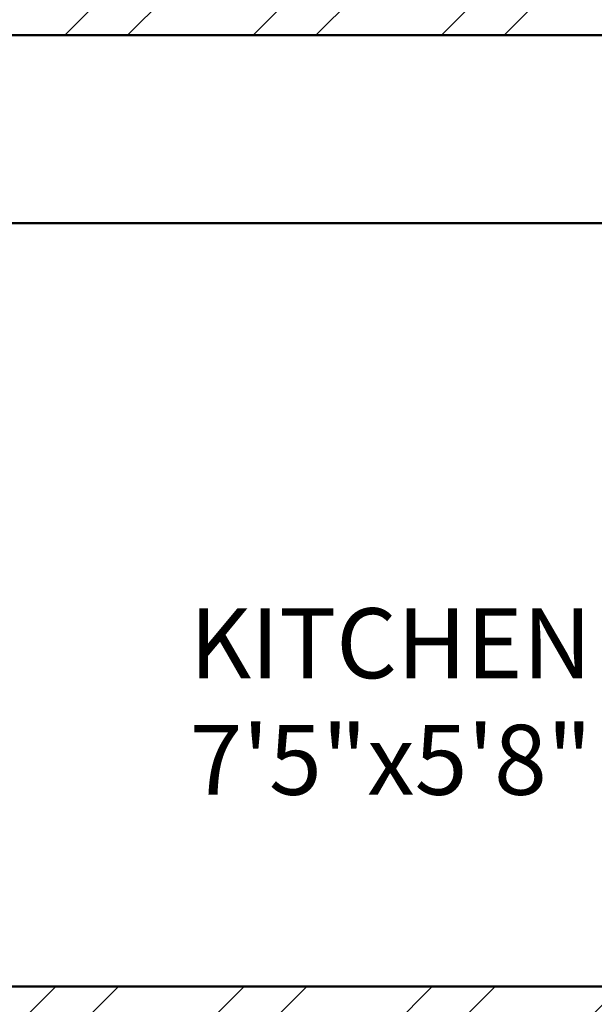
# Model space of a CAD drawing. Units: inches. Extents: x 1901 to 2863, y 888 to 2433.
# Tile 85 of 91: x 2682 to 2723, y 2009 to 2080. Entities that reach past the tile are written whole.
import ezdxf

# ---------------------------------------------------------------- set-up
doc = ezdxf.new("R2010")
doc.units = ezdxf.units.IN
for name, color, linetype, lineweight in [('A-AREA-IDEN', 7, 'Continuous', 18), ('A-WALL', 7, 'Continuous', 50), ('A-WALL-PATT', 8, 'Continuous', 13)]:
    doc.layers.add(name, color=color, linetype=linetype, lineweight=lineweight)
doc.styles.get("Standard").update_dxf_attribs({"font": 'arial.ttf'})

msp = doc.modelspace()

# ---------------------------------------------------------------- hatches: boundary and pattern name
at = {"layer": 'A-WALL-PATT'}
h = msp.add_hatch(dxfattribs=at)
h.set_pattern_fill('ANSI32', color=256)
h.paths.add_polyline_path([(2192.501, 2274.134), (2141.264, 2274.134), (2141.264, 2269.634), (2192.501, 2269.634)])
h.paths.add_polyline_path([(2259.926, 2274.134), (2216.501, 2274.134), (2216.501, 2269.634), (2255.426, 2269.634), (2255.426, 2214.634), (2250.809, 2214.634), (2250.809, 2210.134), (2259.926, 2210.134), (2259.926, 2215.134), (2271.756, 2215.134), (2271.756, 2217.384), (2271.756, 2219.634), (2259.926, 2219.634)])
h.paths.add_polyline_path([(2171.426, 2269.634), (2166.926, 2269.634), (2166.926, 2219.634), (2121.238, 2219.634), (2121.238, 2215.134), (2166.926, 2215.134), (2166.926, 2083.134), (2161.807, 2083.134), (2161.807, 2078.634), (2171.426, 2078.634), (2176.996, 2078.634), (2176.996, 2080.884), (2176.996, 2083.134), (2171.426, 2083.134), (2171.426, 2210.134), (2230.912, 2210.134), (2230.912, 2212.384), (2230.912, 2214.634), (2171.426, 2214.634)])
h.paths.add_polyline_path([(2117.264, 2274.134), (2089.426, 2274.134), (2089.426, 2219.634), (2081.136, 2219.634), (2081.136, 2215.134), (2089.426, 2215.134), (2098.004, 2215.134), (2098.004, 2217.384), (2098.004, 2219.634), (2093.926, 2219.634), (2093.926, 2269.634), (2117.264, 2269.634), (2117.264, 2271.884)])
h.paths.add_polyline_path([(2343.426, 2219.634), (2329.295, 2219.634), (2329.295, 2215.134), (2338.926, 2215.134), (2338.926, 2184.739), (2343.426, 2184.739)])
h.paths.add_polyline_path([(2338.926, 2083.134), (2329.295, 2083.134), (2208.966, 2083.134), (2208.966, 2078.634), (2338.926, 2078.634)])
h.paths.add_polyline_path([(2343.426, 2136.739), (2338.926, 2136.739), (2338.926, 1872.634), (2343.426, 1872.634)])
h.paths.add_polyline_path([(2343.426, 1863.634), (2397.68, 1863.634), (2397.68, 1821.634), (2384.138, 1821.634), (2384.138, 1812.634), (2418.33, 1812.634), (2418.33, 1817.134), (2418.33, 1821.634), (2406.68, 1821.634), (2406.68, 1863.634), (2459.499, 1863.634), (2459.499, 1821.634), (2447.138, 1821.634), (2447.138, 1812.634), (2459.499, 1812.634), (2468.499, 1812.634), (2468.499, 1872.634), (2394.426, 1872.634), (2334.426, 1872.634), (2334.426, 1812.634), (2343.426, 1812.634), (2353.251, 1812.634), (2353.251, 1821.634), (2343.426, 1821.634)])
h.paths.add_polyline_path([(2510.014, 1872.634), (2468.499, 1872.634), (2468.499, 1868.134), (2510.014, 1868.134)])
h.paths.add_polyline_path([(2514.009, 1817.134), (2468.499, 1817.134), (2468.499, 1812.634), (2482.114, 1812.634), (2482.114, 1800.606), (2486.614, 1800.606), (2486.614, 1812.634), (2514.009, 1812.634)])
h.paths.add_polyline_path([(2299.247, 1814.884), (2299.247, 1817.134), (2295.926, 1817.134), (2295.926, 1854.169), (2293.676, 1854.169), (2291.426, 1854.169), (2291.426, 1817.134), (2266.109, 1817.134), (2266.109, 1812.634), (2299.247, 1812.634)])
h.paths.add_polyline_path([(2218.109, 1817.134), (2206.46, 1817.134), (2171.426, 1817.134), (2171.426, 1949.134), (2190.1, 1949.134), (2190.1, 1953.634), (2163.468, 1953.634), (2163.468, 1949.134), (2166.926, 1949.134), (2166.926, 1817.134), (2114.297, 1817.134), (2114.297, 1812.634), (2218.109, 1812.634)])
h.paths.add_polyline_path([(2029.426, 1970.922), (2024.926, 1970.922), (2024.926, 1912.717), (2029.426, 1912.717)])
h.paths.add_polyline_path([(2132.297, 1953.634), (2113.926, 1953.634), (2113.926, 1975.888), (2111.676, 1975.888), (2109.426, 1975.888), (2109.426, 1953.634), (2029.426, 1953.634), (2029.426, 1949.134), (2132.297, 1949.134)])
h.paths.add_polyline_path([(2029.426, 1853.606), (2029.31, 1853.606), (2029.31, 1853.606), (2029.426, 1853.606), (2029.426, 1864.717), (2024.926, 1864.717), (2024.926, 1812.634), (2066.297, 1812.634), (2066.297, 1814.884), (2066.297, 1817.134), (2029.426, 1817.134)])
h.paths.add_polyline_path([(2122.926, 2010.088), (2120.676, 2010.088), (2118.426, 2010.088), (2118.426, 2006.134), (2029.426, 2006.134), (2029.426, 2001.634), (2109.426, 2001.634), (2109.426, 1998.041), (2113.926, 1998.041), (2113.926, 2001.634), (2122.926, 2001.634)])
h.paths.add_polyline_path([(2029.426, 2031.376), (2024.926, 2031.376), (2024.926, 1994.922), (2027.176, 1994.922), (2029.426, 1994.922)])
h.paths.add_polyline_path([(2029.426, 2136.739), (2024.926, 2136.739), (2024.926, 2067.376), (2027.176, 2067.376), (2029.426, 2067.376)])
h.paths.add_polyline_path([(2125.618, 2083.134), (2029.426, 2083.134), (2029.426, 2078.634), (2118.426, 2078.634), (2118.426, 2030.715), (2122.926, 2030.715), (2122.926, 2078.634), (2125.618, 2078.634)])
h.paths.add_polyline_path([(2029.426, 2215.134), (2040.468, 2215.134), (2040.468, 2217.384), (2040.468, 2219.634), (2024.926, 2219.634), (2024.926, 2184.739), (2029.426, 2184.739), (2029.426, 2187.778)])
h.paths.add_polyline_path([(2686.426, 2274.134), (2659.284, 2274.134), (2659.284, 2269.634), (2681.926, 2269.634), (2681.926, 2219.634), (2676.816, 2219.634), (2676.816, 2215.134), (2681.926, 2215.134), (2697.011, 2215.134), (2697.011, 2217.384), (2697.011, 2219.634), (2686.426, 2219.634)])
h.paths.add_polyline_path([(2609.926, 2269.634), (2635.284, 2269.634), (2635.284, 2274.134), (2571.431, 2274.134), (2571.431, 2269.634), (2605.426, 2269.634), (2605.426, 2214.634), (2549.098, 2214.634), (2549.098, 2210.134), (2605.426, 2210.134), (2605.426, 2083.134), (2601.014, 2083.134), (2601.014, 2080.884), (2601.014, 2078.634), (2609.926, 2078.634), (2616.162, 2078.634), (2616.162, 2080.884), (2616.162, 2083.134), (2609.926, 2083.134), (2609.926, 2215.134), (2651.465, 2215.134), (2651.465, 2217.384), (2651.465, 2219.634), (2609.926, 2219.634)])
h.paths.add_polyline_path([(2521.426, 2269.634), (2547.431, 2269.634), (2547.431, 2271.884), (2547.431, 2274.134), (2516.926, 2274.134), (2516.926, 2219.634), (2506.41, 2219.634), (2506.41, 2215.134), (2516.926, 2215.134), (2516.926, 2210.134), (2525.402, 2210.134), (2525.402, 2212.384), (2525.402, 2214.634), (2521.426, 2214.634)])
h.paths.add_polyline_path([(2456.011, 2219.634), (2439.426, 2219.634), (2439.426, 2187.888), (2443.926, 2187.888), (2443.926, 2215.134), (2456.011, 2215.134)])
h.paths.add_polyline_path([(2752.926, 2219.634), (2739.485, 2219.634), (2739.485, 2215.134), (2748.426, 2215.134), (2748.426, 2187.888), (2752.926, 2187.888)])
h.paths.add_polyline_path([(2752.926, 2139.888), (2748.426, 2139.888), (2748.426, 2083.134), (2648.416, 2083.134), (2648.416, 2078.634), (2654.926, 2078.634), (2654.926, 2039.437), (2659.426, 2039.437), (2659.426, 2078.634), (2748.426, 2078.634), (2748.426, 2063.429), (2752.926, 2063.429)])
h.paths.add_polyline_path([(2752.926, 2010.634), (2659.426, 2010.634), (2659.426, 2015.652), (2654.926, 2015.652), (2654.926, 2010.634), (2605.426, 2010.634), (2605.426, 1920.967), (2609.926, 1920.967), (2609.926, 2006.134), (2748.426, 2006.134), (2748.426, 1982.466), (2752.926, 1982.466)])
h.paths.add_polyline_path([(2752.926, 2027.429), (2748.426, 2027.429), (2748.426, 2010.634), (2752.926, 2010.634)])
h.paths.add_polyline_path([(2748.426, 1886.134), (2609.926, 1886.134), (2609.926, 1889.719), (2605.426, 1889.719), (2605.426, 1861.262), (2609.926, 1861.262), (2609.926, 1881.634), (2748.426, 1881.634)])
h.paths.add_polyline_path([(2456.855, 2228.831), (2498.401, 2228.831), (2498.401, 2247.488), (2456.855, 2247.488)], flags=9)
h.paths.add_polyline_path([(2038.602, 2237.418), (2080.174, 2237.418), (2080.174, 2256.075), (2038.602, 2256.075)], flags=9)
h.paths.add_polyline_path([(2292.009, 1062.394), (2539.932, 1062.394), (2539.932, 1099.487), (2292.009, 1099.487)], flags=9)
h.paths.add_polyline_path([(2424.91, 1832.253), (2448.513, 1832.253), (2448.513, 1846.678), (2424.91, 1846.678)], flags=25)
h.paths.add_polyline_path([(2359.076, 1832.253), (2382.678, 1832.253), (2382.678, 1846.678), (2359.076, 1846.678)], flags=25)
h.paths.add_polyline_path([(2352.899, 1684.802), (2367.543, 1684.802), (2367.543, 1697.167), (2352.899, 1697.167)], flags=9)
h.paths.add_polyline_path([(2079.288, 1755.826), (2169.024, 1755.826), (2169.024, 1774.372), (2079.288, 1774.372)], flags=9)
h.paths.add_polyline_path([(2404.09, 1373.857), (2404.09, 1463.593), (2385.544, 1463.593), (2385.544, 1373.857)], flags=9)
h.paths.add_polyline_path([(2268.091, 2236.371), (2309.636, 2236.371), (2309.636, 2255.028), (2268.091, 2255.028)], flags=9)
h.paths.add_polyline_path([(2575.96, 1700.951), (2665.696, 1700.951), (2665.696, 1719.498), (2575.96, 1719.498)], flags=9)
h.paths.add_polyline_path([(2302.962, 1878.474), (2329.524, 1878.474), (2329.524, 1888.777), (2302.962, 1888.777)], flags=9)
h.paths.add_polyline_path([(2097.415, 2240.576), (2126.573, 2240.576), (2126.573, 2259.233), (2097.415, 2259.233)], flags=9)
h.paths.add_polyline_path([(2208.725, 2246.124), (2237.882, 2246.124), (2237.882, 2264.781), (2208.725, 2264.781)], flags=9)
h.paths.add_polyline_path([(2038.147, 1925.958), (2076.987, 1925.958), (2076.987, 1944.615), (2038.147, 1944.615)], flags=9)
h.paths.add_polyline_path([(2239.144, 1926.672), (2288.465, 1926.672), (2288.465, 1945.329), (2239.144, 1945.329)], flags=9)
h.paths.add_polyline_path([(2175.429, 2007.33), (2212.356, 2007.33), (2212.356, 2025.987), (2175.429, 2025.987)], flags=9)
h.paths.add_polyline_path([(2225.034, 2091.794), (2263.875, 2091.794), (2263.875, 2110.451), (2225.034, 2110.451)], flags=9)
h.paths.add_polyline_path([(2035.398, 2098.478), (2074.238, 2098.478), (2074.238, 2117.135), (2035.398, 2117.135)], flags=9)
h.paths.add_polyline_path([(2050.102, 2029.209), (2083.26, 2029.209), (2083.26, 2047.866), (2050.102, 2047.866)], flags=9)
h.paths.add_polyline_path([(2069.677, 1956.719), (2098.835, 1956.719), (2098.835, 1975.376), (2069.677, 1975.376)], flags=25)
h.paths.add_polyline_path([(2328.62, 1753.336), (2361.663, 1753.336), (2361.663, 1771.993), (2328.62, 1771.993)], flags=9)
h.paths.add_polyline_path([(2395.162, 2060.888), (2395.162, 2140.654), (2378.676, 2140.654), (2378.676, 2060.888)], flags=9)
h.paths.add_polyline_path([(2463.728, 2059.02), (2492.886, 2059.02), (2492.886, 2077.677), (2463.728, 2077.677)], flags=9)
h.paths.add_polyline_path([(2458.027, 2181.536), (2496.868, 2181.536), (2496.868, 2200.194), (2458.027, 2200.194)], flags=9)
h.paths.add_polyline_path([(2527.577, 2243.074), (2556.735, 2243.074), (2556.735, 2261.731), (2527.577, 2261.731)], flags=9)
h.paths.add_polyline_path([(2694.461, 2232.767), (2736.033, 2232.767), (2736.033, 2251.425), (2694.461, 2251.425)], flags=9)
h.paths.add_polyline_path([(2637.821, 2249.225), (2666.979, 2249.225), (2666.979, 2267.882), (2637.821, 2267.882)], flags=9)
h.paths.add_polyline_path([(2623.687, 2183.541), (2662.528, 2183.541), (2662.528, 2202.199), (2623.687, 2202.199)], flags=9)
h.paths.add_polyline_path([(2691.965, 2021.5), (2725.124, 2021.5), (2725.124, 2040.157), (2691.965, 2040.157)], flags=9)
h.paths.add_polyline_path([(2621.043, 1975.912), (2662.335, 1975.912), (2662.335, 1994.569), (2621.043, 1994.569)], flags=25)
h.paths.add_polyline_path([(2479.032, 1927.62), (2519.844, 1927.62), (2519.844, 1946.277), (2479.032, 1946.277)], flags=9)
h.paths.add_polyline_path([(2670.941, 1849.076), (2716.005, 1849.076), (2716.005, 1867.734), (2670.941, 1867.734)], flags=9)
h.paths.add_polyline_path([(2523.613, 1782.956), (2550.175, 1782.956), (2550.175, 1793.26), (2523.613, 1793.26)], flags=9)
h.paths.add_polyline_path([(2450.841, 1207.331), (2492.386, 1207.331), (2492.386, 1225.989), (2450.841, 1225.989)], flags=9)
h.paths.add_polyline_path([(2527.751, 1203.841), (2556.908, 1203.841), (2556.908, 1222.499), (2527.751, 1222.499)], flags=9)
h.paths.add_polyline_path([(2639.111, 1207.2), (2668.268, 1207.2), (2668.268, 1225.857), (2639.111, 1225.857)], flags=9)
h.paths.add_polyline_path([(2692.594, 1218.965), (2734.167, 1218.965), (2734.167, 1237.623), (2692.594, 1237.623)], flags=9)
h.paths.add_polyline_path([(2669.266, 1366.329), (2708.106, 1366.329), (2708.106, 1384.987), (2669.266, 1384.987)], flags=9)
h.paths.add_polyline_path([(2463.313, 1358.031), (2502.153, 1358.031), (2502.153, 1376.688), (2463.313, 1376.688)], flags=9)
h.paths.add_polyline_path([(2494.725, 1449.963), (2531.652, 1449.963), (2531.652, 1468.62), (2494.725, 1468.62)], flags=9)
h.paths.add_polyline_path([(2675.565, 1422.157), (2708.724, 1422.157), (2708.724, 1440.815), (2675.565, 1440.815)], flags=9)
h.paths.add_polyline_path([(2685.634, 1493.891), (2714.792, 1493.891), (2714.792, 1512.548), (2685.634, 1512.548)], flags=9)
h.paths.add_polyline_path([(2686.805, 1529.913), (2725.645, 1529.913), (2725.645, 1548.57), (2686.805, 1548.57)], flags=9)
h.paths.add_polyline_path([(2503.651, 1537.991), (2552.972, 1537.991), (2552.972, 1556.648), (2503.651, 1556.648)], flags=9)
h.paths.add_polyline_path([(2291.713, 1643.504), (2318.275, 1643.504), (2318.275, 1653.807), (2291.713, 1653.807)], flags=9)
h.paths.add_polyline_path([(2450.626, 1610.52), (2477.189, 1610.52), (2477.189, 1620.824), (2450.626, 1620.824)], flags=9)
h.paths.add_polyline_path([(2359.985, 1551.814), (2422.253, 1551.814), (2422.253, 1562.117), (2359.985, 1562.117)], flags=9)
h.paths.add_polyline_path([(2280.106, 1249.006), (2321.651, 1249.006), (2321.651, 1267.663), (2280.106, 1267.663)], flags=9)
h.paths.add_polyline_path([(2164.057, 1274.232), (2193.215, 1274.232), (2193.215, 1292.889), (2164.057, 1292.889)], flags=9)
h.paths.add_polyline_path([(2118.21, 1277.694), (2151.252, 1277.694), (2151.252, 1296.351), (2118.21, 1296.351)], flags=9)
h.paths.add_polyline_path([(2031.946, 1268.529), (2073.519, 1268.529), (2073.519, 1287.187), (2031.946, 1287.187)], flags=9)
h.paths.add_polyline_path([(2050.199, 1409.079), (2089.04, 1409.079), (2089.04, 1427.736), (2050.199, 1427.736)], flags=9)
h.paths.add_polyline_path([(2243.743, 1421.032), (2282.584, 1421.032), (2282.584, 1439.689), (2243.743, 1439.689)], flags=9)
h.paths.add_polyline_path([(2190.746, 1509.769), (2231.558, 1509.769), (2231.558, 1528.426), (2190.746, 1528.426)], flags=9)
h.paths.add_polyline_path([(2058.392, 1475.415), (2091.55, 1475.415), (2091.55, 1494.073), (2058.392, 1494.073)], flags=9)
h.paths.add_polyline_path([(2062.447, 1553.09), (2091.605, 1553.09), (2091.605, 1571.747), (2062.447, 1571.747)], flags=9)
h.paths.add_polyline_path([(2219.524, 1590.365), (2266.147, 1590.365), (2266.147, 1609.022), (2219.524, 1609.022)], flags=9)
h.paths.add_polyline_path([(2041.072, 1584.188), (2079.912, 1584.188), (2079.912, 1602.845), (2041.072, 1602.845)], flags=9)
h = msp.add_hatch(dxfattribs=at)
h.set_pattern_fill('ANSI32', color=256)
h.paths.add_polyline_path([(2443.926, 2139.888), (2439.426, 2139.888), (2439.426, 2069.348), (2441.676, 2069.348), (2443.926, 2069.348), (2443.926, 2078.634), (2521.926, 2078.634), (2521.926, 2075.067), (2524.176, 2075.067), (2526.426, 2075.067), (2526.426, 2078.634), (2571.755, 2078.634), (2571.755, 2080.884), (2571.755, 2083.134), (2443.926, 2083.134)])
h.paths.add_polyline_path([(2526.426, 2054.634), (2524.176, 2054.634), (2521.926, 2054.634), (2521.926, 2030.634), (2443.926, 2030.634), (2443.926, 2045.348), (2439.426, 2045.348), (2439.426, 1983.867), (2443.926, 1983.867), (2443.926, 2026.134), (2521.926, 2026.134), (2526.426, 2026.134)])
h.paths.add_polyline_path([(2443.926, 1923.867), (2439.426, 1923.867), (2439.426, 1872.634), (2443.926, 1872.634)])
h.paths.add_polyline_path([(2636.233, 1766.134), (2609.926, 1766.134), (2609.926, 1779.785), (2605.426, 1779.785), (2605.426, 1766.134), (2486.614, 1766.134), (2486.614, 1770.671), (2482.114, 1770.671), (2482.114, 1766.134), (2482.114, 1761.634), (2636.233, 1761.634), (2636.233, 1763.884)])
h.paths.add_polyline_path([(2519.536, 1663.384), (2519.536, 1665.634), (2494.926, 1665.634), (2481.831, 1665.634), (2481.831, 1663.384), (2481.831, 1661.134), (2490.426, 1661.134), (2490.426, 1640.157), (2494.926, 1640.157), (2494.926, 1661.134), (2519.536, 1661.134)])
h.paths.add_polyline_path([(2443.926, 1712.134), (2443.926, 1716.634), (2414.464, 1716.634), (2414.464, 1712.134), (2439.426, 1712.134), (2439.426, 1545.507), (2443.926, 1545.507), (2443.926, 1661.134), (2448.475, 1661.134), (2448.475, 1665.634), (2443.926, 1665.634)])
h.paths.add_polyline_path([(2343.426, 1712.134), (2365.525, 1712.134), (2365.525, 1714.384), (2365.525, 1716.634), (2333.871, 1716.634), (2333.871, 1714.384), (2333.871, 1712.134), (2338.926, 1712.134), (2338.926, 1575.634), (2338.926, 1545.507), (2343.426, 1545.507), (2343.426, 1547.507), (2343.426, 1580.134)])
h.paths.add_polyline_path([(2752.926, 1665.634), (2579.536, 1665.634), (2579.536, 1661.134), (2615.926, 1661.134), (2615.926, 1529.134), (2598.931, 1529.134), (2598.931, 1524.634), (2623.127, 1524.634), (2623.127, 1526.884), (2623.127, 1529.134), (2620.426, 1529.134), (2620.426, 1661.134), (2748.426, 1661.134), (2748.426, 1633.499), (2752.926, 1633.499)])
h.paths.add_polyline_path([(2752.926, 1419.929), (2748.426, 1419.929), (2748.426, 1400.134), (2659.426, 1400.134), (2659.426, 1444.333), (2657.176, 1444.333), (2654.926, 1444.333), (2654.926, 1400.134), (2643.649, 1400.134), (2643.649, 1395.634), (2748.426, 1395.634), (2748.426, 1364.035), (2752.926, 1364.035)])
h.paths.add_polyline_path([(2752.926, 1492.878), (2748.426, 1492.878), (2748.426, 1476.634), (2667.426, 1476.634), (2667.426, 1479.71), (2665.176, 1479.71), (2662.926, 1479.71), (2662.926, 1476.634), (2654.926, 1476.634), (2654.926, 1469.536), (2659.426, 1469.536), (2659.426, 1472.134), (2748.426, 1472.134), (2748.426, 1455.929), (2752.926, 1455.929)])
h.paths.add_polyline_path([(2752.926, 1304.035), (2748.426, 1304.035), (2748.426, 1263.634), (2738.66, 1263.634), (2738.66, 1259.134), (2752.926, 1259.134)])
h.paths.add_polyline_path([(2685.926, 1259.134), (2695.49, 1259.134), (2695.49, 1261.384), (2695.49, 1263.634), (2677.837, 1263.634), (2677.837, 1261.384), (2677.837, 1259.134), (2681.426, 1259.134), (2681.426, 1203.634), (2653.277, 1203.634), (2653.277, 1199.134), (2685.926, 1199.134), (2685.926, 1203.634)])
h.paths.add_polyline_path([(2609.426, 1395.634), (2611.848, 1395.634), (2611.848, 1400.134), (2598.888, 1400.134), (2598.888, 1397.884), (2598.888, 1395.634), (2604.926, 1395.634), (2604.926, 1268.134), (2554.726, 1268.134), (2554.726, 1265.884), (2554.726, 1263.634), (2604.926, 1263.634), (2604.926, 1203.634), (2571.306, 1203.634), (2571.306, 1199.134), (2604.926, 1199.134), (2629.277, 1199.134), (2629.277, 1201.384), (2629.277, 1203.634), (2609.426, 1203.634), (2609.426, 1258.634), (2609.426, 1259.134), (2654.804, 1259.134), (2654.804, 1263.634), (2609.426, 1263.634)])
h.paths.add_polyline_path([(2443.926, 1304.035), (2439.426, 1304.035), (2439.426, 1259.134), (2443.926, 1259.134), (2456.16, 1259.134), (2456.16, 1261.384), (2456.16, 1263.634), (2443.926, 1263.634)])
h.paths.add_polyline_path([(2525.426, 1263.634), (2531.778, 1263.634), (2531.778, 1268.134), (2520.926, 1268.134), (2520.926, 1263.634), (2511.409, 1263.634), (2511.409, 1259.134), (2520.926, 1259.134), (2520.926, 1199.134), (2547.306, 1199.134), (2547.306, 1201.384), (2547.306, 1203.634), (2525.426, 1203.634)])
h.paths.add_polyline_path([(2443.926, 1434.842), (2439.426, 1434.842), (2439.426, 1364.035), (2441.676, 1364.035), (2443.926, 1364.035)])
h.paths.add_polyline_path([(2567.134, 1400.134), (2443.926, 1400.134), (2443.926, 1395.634), (2567.134, 1395.634)])
h.paths.add_polyline_path([(2443.926, 1545.507), (2439.426, 1545.507), (2439.426, 1494.842), (2443.926, 1494.842)])
h.paths.add_polyline_path([(2494.926, 1553.349), (2492.676, 1553.349), (2490.426, 1553.349), (2490.426, 1524.634), (2494.926, 1524.634), (2525.936, 1524.634), (2525.936, 1526.884), (2525.936, 1529.134), (2494.926, 1529.134)])
h.paths.add_polyline_path([(2752.926, 1573.499), (2748.426, 1573.499), (2748.426, 1529.134), (2657.759, 1529.134), (2657.759, 1524.634), (2662.926, 1524.634), (2662.926, 1498.631), (2667.426, 1498.631), (2667.426, 1524.634), (2748.426, 1524.634), (2748.426, 1516.878), (2752.926, 1516.878)])
h.paths.add_polyline_path([(2038.602, 2237.418), (2080.174, 2237.418), (2080.174, 2256.075), (2038.602, 2256.075)], flags=9)
h.paths.add_polyline_path([(2292.009, 1062.394), (2539.932, 1062.394), (2539.932, 1099.487), (2292.009, 1099.487)], flags=9)
h.paths.add_polyline_path([(2424.91, 1832.253), (2448.513, 1832.253), (2448.513, 1846.678), (2424.91, 1846.678)], flags=9)
h.paths.add_polyline_path([(2359.076, 1832.253), (2382.678, 1832.253), (2382.678, 1846.678), (2359.076, 1846.678)], flags=9)
h.paths.add_polyline_path([(2352.899, 1684.802), (2367.543, 1684.802), (2367.543, 1697.167), (2352.899, 1697.167)], flags=9)
h.paths.add_polyline_path([(2079.288, 1755.826), (2169.024, 1755.826), (2169.024, 1774.372), (2079.288, 1774.372)], flags=9)
h.paths.add_polyline_path([(2404.09, 1373.857), (2404.09, 1463.593), (2385.544, 1463.593), (2385.544, 1373.857)], flags=9)
h.paths.add_polyline_path([(2268.091, 2236.371), (2309.636, 2236.371), (2309.636, 2255.028), (2268.091, 2255.028)], flags=9)
h.paths.add_polyline_path([(2575.96, 1700.951), (2665.696, 1700.951), (2665.696, 1719.498), (2575.96, 1719.498)], flags=9)
h.paths.add_polyline_path([(2302.962, 1878.474), (2329.524, 1878.474), (2329.524, 1888.777), (2302.962, 1888.777)], flags=9)
h.paths.add_polyline_path([(2097.415, 2240.576), (2126.573, 2240.576), (2126.573, 2259.233), (2097.415, 2259.233)], flags=9)
h.paths.add_polyline_path([(2208.725, 2246.124), (2237.882, 2246.124), (2237.882, 2264.781), (2208.725, 2264.781)], flags=9)
h.paths.add_polyline_path([(2038.147, 1925.958), (2076.987, 1925.958), (2076.987, 1944.615), (2038.147, 1944.615)], flags=9)
h.paths.add_polyline_path([(2239.144, 1926.672), (2288.465, 1926.672), (2288.465, 1945.329), (2239.144, 1945.329)], flags=9)
h.paths.add_polyline_path([(2175.429, 2007.33), (2212.356, 2007.33), (2212.356, 2025.987), (2175.429, 2025.987)], flags=9)
h.paths.add_polyline_path([(2225.034, 2091.794), (2263.875, 2091.794), (2263.875, 2110.451), (2225.034, 2110.451)], flags=9)
h.paths.add_polyline_path([(2035.398, 2098.478), (2074.238, 2098.478), (2074.238, 2117.135), (2035.398, 2117.135)], flags=9)
h.paths.add_polyline_path([(2050.102, 2029.209), (2083.26, 2029.209), (2083.26, 2047.866), (2050.102, 2047.866)], flags=9)
h.paths.add_polyline_path([(2069.677, 1956.719), (2098.835, 1956.719), (2098.835, 1975.376), (2069.677, 1975.376)], flags=9)
h.paths.add_polyline_path([(2328.62, 1753.336), (2361.663, 1753.336), (2361.663, 1771.993), (2328.62, 1771.993)], flags=9)
h.paths.add_polyline_path([(2395.162, 2060.888), (2395.162, 2140.654), (2378.676, 2140.654), (2378.676, 2060.888)], flags=9)
h.paths.add_polyline_path([(2463.728, 2059.02), (2492.886, 2059.02), (2492.886, 2077.677), (2463.728, 2077.677)], flags=9)
h.paths.add_polyline_path([(2458.027, 2181.536), (2496.868, 2181.536), (2496.868, 2200.194), (2458.027, 2200.194)], flags=9)
h.paths.add_polyline_path([(2456.855, 2228.831), (2498.401, 2228.831), (2498.401, 2247.488), (2456.855, 2247.488)], flags=9)
h.paths.add_polyline_path([(2527.577, 2243.074), (2556.735, 2243.074), (2556.735, 2261.731), (2527.577, 2261.731)], flags=9)
h.paths.add_polyline_path([(2694.461, 2232.767), (2736.033, 2232.767), (2736.033, 2251.425), (2694.461, 2251.425)], flags=9)
h.paths.add_polyline_path([(2637.821, 2249.225), (2666.979, 2249.225), (2666.979, 2267.882), (2637.821, 2267.882)], flags=9)
h.paths.add_polyline_path([(2623.687, 2183.541), (2662.528, 2183.541), (2662.528, 2202.199), (2623.687, 2202.199)], flags=9)
h.paths.add_polyline_path([(2691.965, 2021.5), (2725.124, 2021.5), (2725.124, 2040.157), (2691.965, 2040.157)], flags=9)
h.paths.add_polyline_path([(2621.043, 1975.912), (2662.335, 1975.912), (2662.335, 1994.569), (2621.043, 1994.569)], flags=9)
h.paths.add_polyline_path([(2479.032, 1927.62), (2519.844, 1927.62), (2519.844, 1946.277), (2479.032, 1946.277)], flags=9)
h.paths.add_polyline_path([(2670.941, 1849.076), (2716.005, 1849.076), (2716.005, 1867.734), (2670.941, 1867.734)], flags=9)
h.paths.add_polyline_path([(2523.613, 1782.956), (2550.175, 1782.956), (2550.175, 1793.26), (2523.613, 1793.26)], flags=9)
h.paths.add_polyline_path([(2450.841, 1207.331), (2492.386, 1207.331), (2492.386, 1225.989), (2450.841, 1225.989)], flags=9)
h.paths.add_polyline_path([(2527.751, 1203.841), (2556.908, 1203.841), (2556.908, 1222.499), (2527.751, 1222.499)], flags=9)
h.paths.add_polyline_path([(2639.111, 1207.2), (2668.268, 1207.2), (2668.268, 1225.857), (2639.111, 1225.857)], flags=9)
h.paths.add_polyline_path([(2692.594, 1218.965), (2734.167, 1218.965), (2734.167, 1237.623), (2692.594, 1237.623)], flags=9)
h.paths.add_polyline_path([(2669.266, 1366.329), (2708.106, 1366.329), (2708.106, 1384.987), (2669.266, 1384.987)], flags=25)
h.paths.add_polyline_path([(2463.313, 1358.031), (2502.153, 1358.031), (2502.153, 1376.688), (2463.313, 1376.688)], flags=9)
h.paths.add_polyline_path([(2494.725, 1449.963), (2531.652, 1449.963), (2531.652, 1468.62), (2494.725, 1468.62)], flags=9)
h.paths.add_polyline_path([(2675.565, 1422.157), (2708.724, 1422.157), (2708.724, 1440.815), (2675.565, 1440.815)], flags=25)
h.paths.add_polyline_path([(2685.634, 1493.891), (2714.792, 1493.891), (2714.792, 1512.548), (2685.634, 1512.548)], flags=9)
h.paths.add_polyline_path([(2686.805, 1529.913), (2725.645, 1529.913), (2725.645, 1548.57), (2686.805, 1548.57)], flags=25)
h.paths.add_polyline_path([(2503.651, 1537.991), (2552.972, 1537.991), (2552.972, 1556.648), (2503.651, 1556.648)], flags=9)
h.paths.add_polyline_path([(2291.713, 1643.504), (2318.275, 1643.504), (2318.275, 1653.807), (2291.713, 1653.807)], flags=9)
h.paths.add_polyline_path([(2450.626, 1610.52), (2477.189, 1610.52), (2477.189, 1620.824), (2450.626, 1620.824)], flags=9)
h.paths.add_polyline_path([(2359.985, 1551.814), (2422.253, 1551.814), (2422.253, 1562.117), (2359.985, 1562.117)], flags=9)
h.paths.add_polyline_path([(2280.106, 1249.006), (2321.651, 1249.006), (2321.651, 1267.663), (2280.106, 1267.663)], flags=9)
h.paths.add_polyline_path([(2164.057, 1274.232), (2193.215, 1274.232), (2193.215, 1292.889), (2164.057, 1292.889)], flags=9)
h.paths.add_polyline_path([(2118.21, 1277.694), (2151.252, 1277.694), (2151.252, 1296.351), (2118.21, 1296.351)], flags=9)
h.paths.add_polyline_path([(2031.946, 1268.529), (2073.519, 1268.529), (2073.519, 1287.187), (2031.946, 1287.187)], flags=9)
h.paths.add_polyline_path([(2050.199, 1409.079), (2089.04, 1409.079), (2089.04, 1427.736), (2050.199, 1427.736)], flags=9)
h.paths.add_polyline_path([(2243.743, 1421.032), (2282.584, 1421.032), (2282.584, 1439.689), (2243.743, 1439.689)], flags=9)
h.paths.add_polyline_path([(2190.746, 1509.769), (2231.558, 1509.769), (2231.558, 1528.426), (2190.746, 1528.426)], flags=9)
h.paths.add_polyline_path([(2058.392, 1475.415), (2091.55, 1475.415), (2091.55, 1494.073), (2058.392, 1494.073)], flags=9)
h.paths.add_polyline_path([(2062.447, 1553.09), (2091.605, 1553.09), (2091.605, 1571.747), (2062.447, 1571.747)], flags=9)
h.paths.add_polyline_path([(2219.524, 1590.365), (2266.147, 1590.365), (2266.147, 1609.022), (2219.524, 1609.022)], flags=9)
h.paths.add_polyline_path([(2041.072, 1584.188), (2079.912, 1584.188), (2079.912, 1602.845), (2041.072, 1602.845)], flags=9)

# ---------------------------------------------------------------- linework, layer by layer
at = {"layer": 'A-WALL'}
for p, q in [((2659.426, 2078.634), (2748.426, 2078.634)), ((2659.426, 2065.199), (2734.984, 2065.199)), ((2659.426, 2010.634), (2748.426, 2010.634)), ((2752.926, 2010.634), (2659.426, 2010.634))]:
    msp.add_line(p, q, dxfattribs=at)

# ---------------------------------------------------------------- texts
at = {"layer": 'A-AREA-IDEN', "insert": (2693.727, 2037.669), "char_height": 5, "attachment_point": 1}
msp.add_mtext_dynamic_manual_height_columns('KITCHEN\\P7\'5"x5\'8"', width=113.98684, gutter_width=12.5, heights=[0], dxfattribs=at)

doc.saveas('drawing.dxf')
